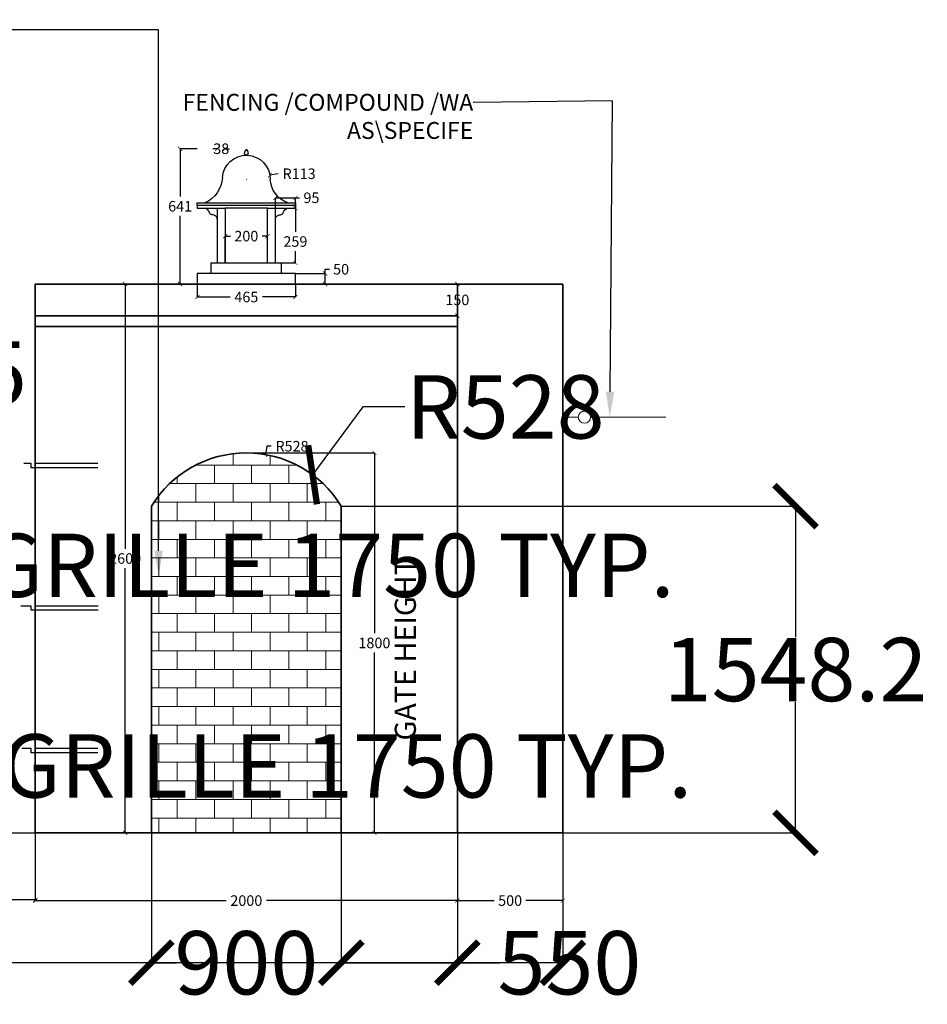
# Model space of a CAD drawing. Units: millimetres. Extents: x 16635 to 28332, y 17519 to 22633.
# Tile 4 of 4: x 24031 to 28332, y 17772 to 22437. Entities that reach past the tile are written whole.
import ezdxf
from ezdxf import colors
from ezdxf.entities.mleader import LeaderData, LeaderLine
from ezdxf.math import Vec2, Vec3

# ---------------------------------------------------------------- set-up
doc = ezdxf.new("R2010")
doc.units = ezdxf.units.MM
doc.header["$MEASUREMENT"] = 0
for name, color, linetype, lineweight in [('A-ANNO-DIMS', 2, 'Continuous', 18), ('A-ANNO-SYMB', 2, 'Continuous', 18), ('A-ANNO-TEXT', 7, 'Continuous', 18), ('A-ELEV-GRAD', 7, 'Continuous', 30), ('A-GATE-HRDW', 3, 'Continuous', 25), ('A-WALL', 7, 'Continuous', 35), ('A-WALL-CHTR', 32, 'Continuous', 25), ('A-WALL-PATT', 8, 'Continuous', 13)]:
    doc.layers.add(name, color=color, linetype=linetype, lineweight=lineweight)
doc.styles.get("Standard").update_dxf_attribs({"font": 'arial.ttf'})
doc.dimstyles.get("Standard").update_dxf_attribs({"dimtxt": 300, "dimasz": 200, "dimexe": 0.18, "dimexo": 0.0625, "dimgap": 0.09, "dimtad": 0, "dimtih": 1, "dimtoh": 1, "dimdec": 0, "dimzin": 0, "dimdsep": 46, "dimtxsty": 'Standard', "dimblk": 'ARCHTICK', "dimcen": 0.09, "dimadec": 0, "dimazin": 0, "dimtfac": 1, "dimtdec": 0, "dimtofl": 0, "dimtmove": 0, "dimatfit": 3, "dimfxl": 1, "dimtolj": 1, "dimtzin": 0, "dimarcsym": 0})

# ---------------------------------------------------------------- blocks, each defined once
blk = doc.blocks.new('_ArchTick')
at = {"color": 0, "linetype": 'ByBlock', "const_width": 0.15}
blk.add_lwpolyline([(-0.5, -0.5), (0.5, 0.5)], dxfattribs=at)
blk = doc.blocks.new('*D1')
at = {"layer": 'A-ANNO-DIMS', "color": 0, "lineweight": -2, "transparency": 16777216}
for p, q in [((25202, 20416), (25195.2, 20376.5)), ((25222, 20416), (25202, 20416)), ((25104.7, 19856.3), (25104.9, 19856.3)), ((25104.8, 19856.3), (25104.8, 19856.4))]:
    blk.add_line(p, q, dxfattribs=at)
at = {"layer": 'Defpoints', "color": 0, "transparency": 16777216}
for p in [(25195.2, 20376.5), (25104.8, 19856.3)]:
    blk.add_point(p, dxfattribs=at)
at = {"layer": 'A-ANNO-DIMS', "color": 0, "lineweight": -2, "transparency": 16777216, "xscale": 20, "yscale": 20, "zscale": 20, "rotation": 260.1400745692449}
blk.add_blockref('_ArchTick', (25195.2, 20376.5), dxfattribs=at)
at = {"layer": 'A-ANNO-DIMS', "color": 0, "transparency": 16777216, "insert": (25321.2, 20416), "char_height": 50, "attachment_point": 5}
blk.add_mtext('\\A1;R528', dxfattribs=at)
blk = doc.blocks.new('*D2')
at = {"layer": 'A-ANNO-DIMS', "color": 0, "lineweight": -2, "transparency": 16777216}
for p, q in [((24872.2, 21825.3), (24790.9, 21825.3)), ((24791.1, 21825.3), (24791.1, 21598.3)), ((24791.1, 21184.3), (24791.1, 21507.3)), ((24872.2, 21184.3), (24790.9, 21184.3))]:
    blk.add_line(p, q, dxfattribs=at)
at = {"layer": 'Defpoints', "color": 0, "transparency": 16777216}
for p in [(24791.1, 21825.3), (24872.3, 21825.3), (24872.3, 21184.3)]:
    blk.add_point(p, dxfattribs=at)
at = {"layer": 'A-ANNO-DIMS', "color": 0, "lineweight": -2, "transparency": 16777216, "xscale": 20, "yscale": 20, "zscale": 20}
for p, rotation in [((24791.1, 21825.3), 90), ((24791.1, 21184.3), 270)]:
    blk.add_blockref('_ArchTick', p, dxfattribs=dict(at, rotation=rotation))
at = {"layer": 'A-ANNO-DIMS', "color": 0, "transparency": 16777216, "insert": (24791.1, 21552.8), "char_height": 50, "attachment_point": 5}
blk.add_mtext('\\A1;641', dxfattribs=at)
blk = doc.blocks.new('*D3')
at = {"layer": 'A-ANNO-DIMS', "color": 0, "lineweight": -2, "transparency": 16777216}
for p, q in [((25255.6, 21706.8), (25216.2, 21700.2)), ((25104.7, 21681.3), (25104.9, 21681.3)), ((25104.8, 21681.3), (25104.8, 21681.4))]:
    blk.add_line(p, q, dxfattribs=at)
at = {"layer": 'Defpoints', "color": 0, "transparency": 16777216}
for p in [(25216.2, 21700.2), (25104.8, 21681.3)]:
    blk.add_point(p, dxfattribs=at)
at = {"layer": 'A-ANNO-DIMS', "color": 0, "lineweight": -2, "transparency": 16777216, "xscale": 20, "yscale": 20, "zscale": 20, "rotation": 189.582500647435}
blk.add_blockref('_ArchTick', (25216.2, 21700.2), dxfattribs=at)
at = {"layer": 'A-ANNO-DIMS', "color": 0, "transparency": 16777216, "insert": (25354.8, 21706.8), "char_height": 50, "attachment_point": 5}
blk.add_mtext('\\A1;R113', dxfattribs=at)
blk = doc.blocks.new('*D4')
at = {"layer": 'A-ANNO-DIMS', "color": 0, "lineweight": -2, "transparency": 16777216}
for p, q in [((24966.8, 21825.3), (24946.8, 21825.3)), ((24966.8, 21825.4), (24966.8, 21825.5)), ((25004.8, 21825.4), (25004.8, 21825.5)), ((25004.8, 21825.3), (25024.8, 21825.3))]:
    blk.add_line(p, q, dxfattribs=at)
at = {"layer": 'Defpoints', "color": 0, "transparency": 16777216}
for p in [(24966.8, 21825.3), (25004.8, 21825.3), (25004.8, 21825.3)]:
    blk.add_point(p, dxfattribs=at)
at = {"layer": 'A-ANNO-DIMS', "color": 0, "lineweight": -2, "transparency": 16777216, "xscale": 20, "yscale": 20, "zscale": 20}
blk.add_blockref('_ArchTick', (24966.8, 21825.3), dxfattribs=at)
at = {"layer": 'A-ANNO-DIMS', "color": 0, "lineweight": -2, "transparency": 16777216, "xscale": 20, "yscale": 20, "zscale": 20, "rotation": 180}
blk.add_blockref('_ArchTick', (25004.8, 21825.3), dxfattribs=at)
at = {"layer": 'A-ANNO-DIMS', "color": 0, "transparency": 16777216, "insert": (24985.8, 21825.3), "char_height": 50, "attachment_point": 5}
blk.add_mtext('\\A1;38', dxfattribs=at)
blk = doc.blocks.new('*D5')
at = {"layer": 'A-ANNO-DIMS', "color": 0, "lineweight": -2, "transparency": 16777216}
for p, q in [((25004.8, 21284.4), (25004.8, 21411.5)), ((25004.8, 21411.3), (25029.2, 21411.3)), ((25204.8, 21411.3), (25180.3, 21411.3)), ((25204.8, 21284.4), (25204.8, 21411.5))]:
    blk.add_line(p, q, dxfattribs=at)
at = {"layer": 'Defpoints', "color": 0, "transparency": 16777216}
for p in [(25204.8, 21411.3), (25004.8, 21284.3), (25204.8, 21284.3)]:
    blk.add_point(p, dxfattribs=at)
at = {"layer": 'A-ANNO-DIMS', "color": 0, "lineweight": -2, "transparency": 16777216, "xscale": 20, "yscale": 20, "zscale": 20, "rotation": 180}
blk.add_blockref('_ArchTick', (25004.8, 21411.3), dxfattribs=at)
at = {"layer": 'A-ANNO-DIMS', "color": 0, "lineweight": -2, "transparency": 16777216, "xscale": 20, "yscale": 20, "zscale": 20}
blk.add_blockref('_ArchTick', (25204.8, 21411.3), dxfattribs=at)
at = {"layer": 'A-ANNO-DIMS', "color": 0, "transparency": 16777216, "insert": (25104.8, 21411.3), "char_height": 50, "attachment_point": 5}
blk.add_mtext('\\A1;200', dxfattribs=at)
blk = doc.blocks.new('*D6')
at = {"layer": 'A-ANNO-DIMS', "color": 0, "lineweight": -2, "transparency": 16777216}
for p, q in [((25337.3, 21234.3), (25478.4, 21234.3)), ((25478.2, 21234.3), (25478.2, 21254.3)), ((25478.2, 21254.3), (25498.2, 21254.3)), ((25478.2, 21184.3), (25478.2, 21234.3)), ((25337.3, 21184.3), (25478.4, 21184.3))]:
    blk.add_line(p, q, dxfattribs=at)
at = {"layer": 'Defpoints', "color": 0, "transparency": 16777216}
for p in [(25337.3, 21234.3), (25478.2, 21234.3), (25337.3, 21184.3)]:
    blk.add_point(p, dxfattribs=at)
at = {"layer": 'A-ANNO-DIMS', "color": 0, "lineweight": -2, "transparency": 16777216, "xscale": 20, "yscale": 20, "zscale": 20}
for p, rotation in [((25478.2, 21234.3), 90), ((25478.2, 21184.3), 270)]:
    blk.add_blockref('_ArchTick', p, dxfattribs=dict(at, rotation=rotation))
at = {"layer": 'A-ANNO-DIMS', "color": 0, "transparency": 16777216, "insert": (25553.9, 21254.3), "char_height": 50, "attachment_point": 5}
blk.add_mtext('\\A1;50', dxfattribs=at)
blk = doc.blocks.new('*D7')
at = {"layer": 'A-ANNO-DIMS', "color": 0, "lineweight": -2, "transparency": 16777216}
for p, q in [((24104.8, 21184.3), (24530.8, 21184.3)), ((24530.6, 21184.3), (24530.6, 19929.9)), ((24530.6, 18584.3), (24530.6, 19838.8)), ((24104.8, 18584.3), (24530.8, 18584.3))]:
    blk.add_line(p, q, dxfattribs=at)
at = {"layer": 'Defpoints', "color": 0, "transparency": 16777216}
for p in [(24104.8, 21184.3), (24104.8, 18584.3), (24530.6, 18584.3)]:
    blk.add_point(p, dxfattribs=at)
at = {"layer": 'A-ANNO-DIMS', "color": 0, "lineweight": -2, "transparency": 16777216, "xscale": 20, "yscale": 20, "zscale": 20}
for p, rotation in [((24530.6, 21184.3), 90), ((24530.6, 18584.3), 270)]:
    blk.add_blockref('_ArchTick', p, dxfattribs=dict(at, rotation=rotation))
at = {"layer": 'A-ANNO-DIMS', "color": 0, "transparency": 16777216, "insert": (24530.6, 19884.3), "char_height": 50, "attachment_point": 5}
blk.add_mtext('\\A1;2600', dxfattribs=at)
blk = doc.blocks.new('*D19')
at = {"layer": 'A-ANNO-DIMS', "color": 0, "lineweight": -2, "transparency": 16777216}
for p, q in [((20204.8, 18584.3), (20204.8, 18267)), ((24104.8, 18584.3), (24104.8, 18267)), ((20204.8, 18267.2), (22060.2, 18267.2)), ((24104.8, 18267.2), (22249.3, 18267.2))]:
    blk.add_line(p, q, dxfattribs=at)
at = {"layer": 'Defpoints', "color": 0, "transparency": 16777216}
for p in [(20204.8, 18584.3), (24104.8, 18584.3), (24104.8, 18267.2)]:
    blk.add_point(p, dxfattribs=at)
at = {"layer": 'A-ANNO-DIMS', "color": 0, "lineweight": -2, "transparency": 16777216, "xscale": 20, "yscale": 20, "zscale": 20, "rotation": 180}
blk.add_blockref('_ArchTick', (20204.8, 18267.2), dxfattribs=at)
at = {"layer": 'A-ANNO-DIMS', "color": 0, "lineweight": -2, "transparency": 16777216, "xscale": 20, "yscale": 20, "zscale": 20}
blk.add_blockref('_ArchTick', (24104.8, 18267.2), dxfattribs=at)
at = {"layer": 'A-ANNO-DIMS', "color": 0, "transparency": 16777216, "insert": (22154.8, 18267.2), "char_height": 50, "attachment_point": 5}
blk.add_mtext('\\A1;3900', dxfattribs=at)
blk = doc.blocks.new('*D20')
at = {"layer": 'A-ANNO-DIMS', "color": 0, "lineweight": -2, "transparency": 16777216}
for p, q in [((24104.8, 18584.3), (24104.8, 18263.6)), ((26104.8, 18584.3), (26104.8, 18263.6)), ((24104.8, 18263.8), (25009.8, 18263.8)), ((26104.8, 18263.8), (25199.8, 18263.8))]:
    blk.add_line(p, q, dxfattribs=at)
at = {"layer": 'Defpoints', "color": 0, "transparency": 16777216}
for p in [(24104.8, 18584.3), (26104.8, 18584.3), (26104.8, 18263.8)]:
    blk.add_point(p, dxfattribs=at)
at = {"layer": 'A-ANNO-DIMS', "color": 0, "lineweight": -2, "transparency": 16777216, "xscale": 20, "yscale": 20, "zscale": 20, "rotation": 180}
blk.add_blockref('_ArchTick', (24104.8, 18263.8), dxfattribs=at)
at = {"layer": 'A-ANNO-DIMS', "color": 0, "lineweight": -2, "transparency": 16777216, "xscale": 20, "yscale": 20, "zscale": 20}
blk.add_blockref('_ArchTick', (26104.8, 18263.8), dxfattribs=at)
at = {"layer": 'A-ANNO-DIMS', "color": 0, "transparency": 16777216, "insert": (25104.8, 18263.8), "char_height": 50, "attachment_point": 5}
blk.add_mtext('\\A1;2000', dxfattribs=at)
blk = doc.blocks.new('*D21')
at = {"layer": 'A-ANNO-DIMS', "color": 0, "lineweight": -2, "transparency": 16777216}
for p, q in [((26104.8, 18584.3), (26104.8, 18263.6)), ((26604.8, 18584.3), (26604.8, 18263.6)), ((26104.8, 18263.8), (26279.6, 18263.8)), ((26604.8, 18263.8), (26429.9, 18263.8))]:
    blk.add_line(p, q, dxfattribs=at)
at = {"layer": 'Defpoints', "color": 0, "transparency": 16777216}
for p in [(26104.8, 18584.3), (26604.8, 18584.3), (26604.8, 18263.8)]:
    blk.add_point(p, dxfattribs=at)
at = {"layer": 'A-ANNO-DIMS', "color": 0, "lineweight": -2, "transparency": 16777216, "xscale": 20, "yscale": 20, "zscale": 20, "rotation": 180}
blk.add_blockref('_ArchTick', (26104.8, 18263.8), dxfattribs=at)
at = {"layer": 'A-ANNO-DIMS', "color": 0, "lineweight": -2, "transparency": 16777216, "xscale": 20, "yscale": 20, "zscale": 20}
blk.add_blockref('_ArchTick', (26604.8, 18263.8), dxfattribs=at)
at = {"layer": 'A-ANNO-DIMS', "color": 0, "transparency": 16777216, "insert": (26354.8, 18263.8), "char_height": 50, "attachment_point": 5}
blk.add_mtext('\\A1;500', dxfattribs=at)
blk = doc.blocks.new('*D22')
at = {"layer": 'A-ANNO-DIMS', "color": 0, "lineweight": -2, "transparency": 16777216}
for p, q in [((25104.8, 20384.3), (25711.9, 20384.3)), ((25711.8, 20384.3), (25711.8, 19529.9)), ((25711.8, 18584.3), (25711.8, 19438.8)), ((25104.8, 18584.3), (25711.9, 18584.3))]:
    blk.add_line(p, q, dxfattribs=at)
at = {"layer": 'Defpoints', "color": 0, "transparency": 16777216}
for p in [(25104.8, 20384.3), (25104.8, 18584.3), (25711.8, 18584.3)]:
    blk.add_point(p, dxfattribs=at)
at = {"layer": 'A-ANNO-DIMS', "color": 0, "lineweight": -2, "transparency": 16777216, "xscale": 20, "yscale": 20, "zscale": 20}
for p, rotation in [((25711.8, 20384.3), 90), ((25711.8, 18584.3), 270)]:
    blk.add_blockref('_ArchTick', p, dxfattribs=dict(at, rotation=rotation))
at = {"layer": 'A-ANNO-DIMS', "color": 0, "transparency": 16777216, "insert": (25711.8, 19484.3), "char_height": 50, "attachment_point": 5}
blk.add_mtext('\\A1;1800', dxfattribs=at)
blk = doc.blocks.new('*D25')
at = {"layer": 'A-ANNO-DIMS', "color": 0, "lineweight": -2, "transparency": 16777216}
for p, q in [((26104.7, 21184.3), (26104.6, 21184.3)), ((26104.8, 21184.3), (26104.8, 21154.9)), ((26104.8, 21034.3), (26104.8, 21063.8)), ((26104.7, 21034.3), (26104.6, 21034.3))]:
    blk.add_line(p, q, dxfattribs=at)
at = {"layer": 'Defpoints', "color": 0, "transparency": 16777216}
for p in [(26104.8, 21184.3), (26104.8, 21034.3), (26104.8, 21034.3)]:
    blk.add_point(p, dxfattribs=at)
at = {"layer": 'A-ANNO-DIMS', "color": 0, "lineweight": -2, "transparency": 16777216, "xscale": 20, "yscale": 20, "zscale": 20}
for p, rotation in [((26104.8, 21184.3), 90), ((26104.8, 21034.3), 270)]:
    blk.add_blockref('_ArchTick', p, dxfattribs=dict(at, rotation=rotation))
at = {"layer": 'A-ANNO-DIMS', "color": 0, "transparency": 16777216, "insert": (26104.8, 21109.3), "char_height": 50, "attachment_point": 5}
blk.add_mtext('\\A1;150', dxfattribs=at)
blk = doc.blocks.new('*D26')
at = {"layer": 'A-ANNO-DIMS', "color": 0, "lineweight": -2, "transparency": 16777216}
for p, q in [((24872.3, 21184.3), (24872.3, 21122.9)), ((25337.3, 21184.3), (25337.3, 21122.9)), ((24872.3, 21123), (25028.3, 21123)), ((25337.3, 21123), (25181.2, 21123))]:
    blk.add_line(p, q, dxfattribs=at)
at = {"layer": 'Defpoints', "color": 0, "transparency": 16777216}
for p in [(24872.3, 21184.3), (25337.3, 21184.3), (25337.3, 21123)]:
    blk.add_point(p, dxfattribs=at)
at = {"layer": 'A-ANNO-DIMS', "color": 0, "lineweight": -2, "transparency": 16777216, "xscale": 20, "yscale": 20, "zscale": 20, "rotation": 180}
blk.add_blockref('_ArchTick', (24872.3, 21123), dxfattribs=at)
at = {"layer": 'A-ANNO-DIMS', "color": 0, "lineweight": -2, "transparency": 16777216, "xscale": 20, "yscale": 20, "zscale": 20}
blk.add_blockref('_ArchTick', (25337.3, 21123), dxfattribs=at)
at = {"layer": 'A-ANNO-DIMS', "color": 0, "transparency": 16777216, "insert": (25104.8, 21123), "char_height": 50, "attachment_point": 5}
blk.add_mtext('\\A1;465', dxfattribs=at)
blk = doc.blocks.new('*D27')
at = {"layer": 'A-ANNO-DIMS', "color": 0, "lineweight": -2, "transparency": 16777216}
for p, q in [((25242.8, 21543.4), (25242.8, 21593.1)), ((25242.8, 21593), (25337.3, 21593)), ((25337.3, 21543.4), (25337.3, 21593.1)), ((25337.3, 21593), (25357.3, 21593))]:
    blk.add_line(p, q, dxfattribs=at)
at = {"layer": 'Defpoints', "color": 0, "transparency": 16777216}
for p in [(25337.3, 21593), (25242.8, 21543.3), (25337.3, 21543.3)]:
    blk.add_point(p, dxfattribs=at)
at = {"layer": 'A-ANNO-DIMS', "color": 0, "lineweight": -2, "transparency": 16777216, "xscale": 20, "yscale": 20, "zscale": 20, "rotation": 180}
blk.add_blockref('_ArchTick', (25242.8, 21593), dxfattribs=at)
at = {"layer": 'A-ANNO-DIMS', "color": 0, "lineweight": -2, "transparency": 16777216, "xscale": 20, "yscale": 20, "zscale": 20}
blk.add_blockref('_ArchTick', (25337.3, 21593), dxfattribs=at)
at = {"layer": 'A-ANNO-DIMS', "color": 0, "transparency": 16777216, "insert": (25413.3, 21593), "char_height": 50, "attachment_point": 5}
blk.add_mtext('\\A1;95', dxfattribs=at)
blk = doc.blocks.new('*D29')
at = {"layer": 'A-ANNO-DIMS', "color": 0, "lineweight": -2, "transparency": 16777216}
for p, q in [((25204.8, 21543.3), (25337.5, 21543.3)), ((25337.3, 21543.3), (25337.3, 21431.2)), ((25337.3, 21284.3), (25337.3, 21340.2)), ((25204.8, 21284.3), (25337.5, 21284.3))]:
    blk.add_line(p, q, dxfattribs=at)
at = {"layer": 'Defpoints', "color": 0, "transparency": 16777216}
for p in [(25204.8, 21543.3), (25204.8, 21284.3), (25337.3, 21284.3)]:
    blk.add_point(p, dxfattribs=at)
at = {"layer": 'A-ANNO-DIMS', "color": 0, "lineweight": -2, "transparency": 16777216, "xscale": 20, "yscale": 20, "zscale": 20}
for p, rotation in [((25337.3, 21543.3), 90), ((25337.3, 21284.3), 270)]:
    blk.add_blockref('_ArchTick', p, dxfattribs=dict(at, rotation=rotation))
at = {"layer": 'A-ANNO-DIMS', "color": 0, "transparency": 16777216, "insert": (25337.3, 21385.7), "char_height": 50, "attachment_point": 5}
blk.add_mtext('\\A1;259', dxfattribs=at)
blk = doc.blocks.new('STONE-CHHATRI-ELEV')
for p, q in [((465, 384), (0, 384)), ((0, 384), (0, 359)), ((465, 371.5), (465, 384)), ((0, 371.5), (465, 371.5)), ((132.5, 359), (0, 359)), ((94.5, 100), (94.5, 359)), ((132.5, 100), (132.5, 359)), ((132.5, 359), (332.5, 359)), ((332.5, 359), (332.5, 100)), ((465, 359), (332.5, 359)), ((370.5, 359), (370.5, 100)), ((465, 371.5), (465, 359)), ((398.8, 100), (66.3, 100)), ((66.3, 50), (66.3, 100)), ((398.8, 50), (398.8, 100)), ((0, 0), (0, 50)), ((0, 50), (465, 50)), ((465, 50), (465, 0))]:
    blk.add_line(p, q)
for points in [[(223.5, 618.7, -0.258687), (233, 636.9, -0.244698), (241.5, 619.3, -0.244698)], [(94.5, 307.9, 0.449164), (70.8, 327.5, -0.238561), (57.7, 338.5, 0.309009), (37.1, 359, -1.219644)], [(370.5, 307.9, -0.449164), (394.2, 327.5, 0.238561), (407.3, 338.5, -0.309009), (427.9, 359, 1.219644)]]:
    blk.add_lwpolyline(points, format="xyb")
for centre, radius, start, end in [((232.5, 497), 113, 3.6245, 179.9064), ((232.5, 619), 9.02, 180.1799, 1.9928), ((-8.8, 504.3), 128.5, 290.6287, 356.8247), ((488.3, 514.4), 143.4, 184.0947, 245.367)]:
    blk.add_arc(centre, radius, start, end)
blk = doc.blocks.new('GATE-JAMB-ANCHOR-SET')
for p, q in [((0.2, 1370), (297.2, 1370)), ((317.2, 1350), (317.2, 1370)), ((317.2, 1370), (351.9, 1370)), ((0.2, 1350), (297.2, 1350)), ((297.2, 1350), (317.2, 1350)), ((0, 694.8), (297, 694.8)), ((0, 674.8), (297, 674.8)), ((297, 674.8), (317, 674.8)), ((317, 674.8), (317, 694.8)), ((317, 694.8), (365.3, 694.8)), ((0.2, 20), (297.2, 20)), ((317.2, 0), (317.2, 20)), ((317.2, 20), (360.9, 20)), ((0.2, 0), (297.2, 0)), ((297.2, 0), (317.2, 0))]:
    blk.add_line(p, q)
blk = doc.blocks.new('*D43')
at = {"layer": 'A-ANNO-DIMS', "color": 0, "lineweight": -2, "transparency": 16777216}
for p, q in [((20304.8, 19164.3), (20304.8, 18901.7)), ((22054.8, 19164.3), (22054.8, 18901.7)), ((20304.8, 18901.8), (22054.8, 18901.8)), ((22054.8, 18901.8), (22254.8, 18901.8))]:
    blk.add_line(p, q, dxfattribs=at)
at = {"layer": 'Defpoints', "color": 0, "transparency": 16777216}
for p in [(20304.8, 19164.3), (22054.8, 19164.3), (22054.8, 18901.8)]:
    blk.add_point(p, dxfattribs=at)
at = {"layer": 'A-ANNO-DIMS', "color": 0, "lineweight": -2, "transparency": 16777216, "xscale": 200, "yscale": 200, "zscale": 200, "rotation": 180}
blk.add_blockref('_ArchTick', (20304.8, 18901.8), dxfattribs=at)
at = {"layer": 'A-ANNO-DIMS', "color": 0, "lineweight": -2, "transparency": 16777216, "xscale": 200, "yscale": 200, "zscale": 200}
blk.add_blockref('_ArchTick', (22054.8, 18901.8), dxfattribs=at)
at = {"layer": 'A-ANNO-DIMS', "color": 0, "transparency": 16777216, "insert": (24841.7, 18901.8), "char_height": 300, "attachment_point": 5}
blk.add_mtext('\\A1;LOWER GRILLE 1750 TYP.', dxfattribs=at)
blk = doc.blocks.new('*D45')
at = {"layer": 'A-ANNO-DIMS', "color": 0, "lineweight": -2, "transparency": 16777216}
for p, q in [((20304.8, 20114.3), (20304.8, 19851.7)), ((22054.8, 20114.3), (22054.8, 19851.7)), ((20304.8, 19851.8), (22054.8, 19851.8)), ((22054.8, 19851.8), (22254.8, 19851.8))]:
    blk.add_line(p, q, dxfattribs=at)
at = {"layer": 'Defpoints', "color": 0, "transparency": 16777216}
for p in [(20304.8, 20114.3), (22054.8, 20114.3), (22054.8, 19851.8)]:
    blk.add_point(p, dxfattribs=at)
at = {"layer": 'A-ANNO-DIMS', "color": 0, "lineweight": -2, "transparency": 16777216, "xscale": 200, "yscale": 200, "zscale": 200, "rotation": 180}
blk.add_blockref('_ArchTick', (20304.8, 19851.8), dxfattribs=at)
at = {"layer": 'A-ANNO-DIMS', "color": 0, "lineweight": -2, "transparency": 16777216, "xscale": 200, "yscale": 200, "zscale": 200}
blk.add_blockref('_ArchTick', (22054.8, 19851.8), dxfattribs=at)
at = {"layer": 'A-ANNO-DIMS', "color": 0, "transparency": 16777216, "insert": (24794.1, 19851.8), "char_height": 300, "attachment_point": 5}
blk.add_mtext('\\A1;UPPER GRILLE 1750 TYP.', dxfattribs=at)
blk = doc.blocks.new('*D51')
at = {"layer": 'A-ANNO-DIMS', "color": 0, "lineweight": -2, "transparency": 16777216}
for p, q in [((17704.8, 18584.3), (17704.8, 17969.2)), ((26604.8, 18584.3), (26604.8, 17969.2)), ((17704.8, 17969.3), (21707, 17969.3)), ((26604.8, 17969.3), (22602.5, 17969.3))]:
    blk.add_line(p, q, dxfattribs=at)
at = {"layer": 'Defpoints', "color": 0, "transparency": 16777216}
for p in [(17704.8, 18584.3), (26604.8, 18584.3), (26604.8, 17969.3)]:
    blk.add_point(p, dxfattribs=at)
at = {"layer": 'A-ANNO-DIMS', "color": 0, "lineweight": -2, "transparency": 16777216, "xscale": 200, "yscale": 200, "zscale": 200, "rotation": 180}
blk.add_blockref('_ArchTick', (17704.8, 17969.3), dxfattribs=at)
at = {"layer": 'A-ANNO-DIMS', "color": 0, "lineweight": -2, "transparency": 16777216, "xscale": 200, "yscale": 200, "zscale": 200}
blk.add_blockref('_ArchTick', (26604.8, 17969.3), dxfattribs=at)
at = {"layer": 'A-ANNO-DIMS', "color": 0, "transparency": 16777216, "insert": (22154.8, 17969.3), "char_height": 300, "attachment_point": 5}
blk.add_mtext('\\A1;8900', dxfattribs=at)
blk = doc.blocks.new('*D54')
at = {"layer": 'A-ANNO-DIMS', "color": 0, "lineweight": -2, "transparency": 16777216}
for p, q in [((25554.8, 20132.5), (27707.3, 20132.5)), ((27707.2, 20132.5), (27707.2, 19511.7)), ((27707.2, 18584.3), (27707.2, 19205.2)), ((25554.8, 18584.3), (27707.3, 18584.3))]:
    blk.add_line(p, q, dxfattribs=at)
at = {"layer": 'Defpoints', "color": 0, "transparency": 16777216}
for p in [(25554.8, 20132.5), (27707.2, 20132.5), (25554.8, 18584.3)]:
    blk.add_point(p, dxfattribs=at)
at = {"layer": 'A-ANNO-DIMS', "color": 0, "lineweight": -2, "transparency": 16777216, "xscale": 200, "yscale": 200, "zscale": 200}
for p, rotation in [((27707.2, 20132.5), 90), ((27707.2, 18584.3), 270)]:
    blk.add_blockref('_ArchTick', p, dxfattribs=dict(at, rotation=rotation))
at = {"layer": 'A-ANNO-DIMS', "color": 0, "transparency": 16777216, "insert": (27707.2, 19358.4), "char_height": 300, "attachment_point": 5}
blk.add_mtext('\\A1;1548.2', dxfattribs=at)
blk = doc.blocks.new('*D57')
at = {"layer": 'A-ANNO-DIMS', "color": 0, "lineweight": -2, "transparency": 16777216}
for p, q in [((25554.8, 18584.3), (25554.8, 17969.2)), ((26104.8, 18584.3), (26104.8, 17969.2)), ((25554.8, 17969.3), (26104.8, 17969.3)), ((26104.8, 17969.3), (26304.8, 17969.3))]:
    blk.add_line(p, q, dxfattribs=at)
at = {"layer": 'Defpoints', "color": 0, "transparency": 16777216}
for p in [(25554.8, 18584.3), (26104.8, 18584.3), (26104.8, 17969.3)]:
    blk.add_point(p, dxfattribs=at)
at = {"layer": 'A-ANNO-DIMS', "color": 0, "lineweight": -2, "transparency": 16777216, "xscale": 200, "yscale": 200, "zscale": 200, "rotation": 180}
blk.add_blockref('_ArchTick', (25554.8, 17969.3), dxfattribs=at)
at = {"layer": 'A-ANNO-DIMS', "color": 0, "lineweight": -2, "transparency": 16777216, "xscale": 200, "yscale": 200, "zscale": 200}
blk.add_blockref('_ArchTick', (26104.8, 17969.3), dxfattribs=at)
at = {"layer": 'A-ANNO-DIMS', "color": 0, "transparency": 16777216, "insert": (26635.8, 17969.3), "char_height": 300, "attachment_point": 5}
blk.add_mtext('\\A1;550', dxfattribs=at)
blk = doc.blocks.new('*D58')
at = {"layer": 'A-ANNO-DIMS', "color": 0, "lineweight": -2, "transparency": 16777216}
for p, q in [((24654.8, 18584.3), (24654.8, 17969.2)), ((25554.8, 18584.3), (25554.8, 17969.2)), ((24654.8, 17969.3), (24773.8, 17969.3)), ((25554.8, 17969.3), (25435.8, 17969.3))]:
    blk.add_line(p, q, dxfattribs=at)
at = {"layer": 'Defpoints', "color": 0, "transparency": 16777216}
for p in [(24654.8, 18584.3), (25554.8, 18584.3), (25554.8, 17969.3)]:
    blk.add_point(p, dxfattribs=at)
at = {"layer": 'A-ANNO-DIMS', "color": 0, "lineweight": -2, "transparency": 16777216, "xscale": 200, "yscale": 200, "zscale": 200, "rotation": 180}
blk.add_blockref('_ArchTick', (24654.8, 17969.3), dxfattribs=at)
at = {"layer": 'A-ANNO-DIMS', "color": 0, "lineweight": -2, "transparency": 16777216, "xscale": 200, "yscale": 200, "zscale": 200}
blk.add_blockref('_ArchTick', (25554.8, 17969.3), dxfattribs=at)
at = {"layer": 'A-ANNO-DIMS', "color": 0, "transparency": 16777216, "insert": (25104.8, 17969.3), "char_height": 300, "attachment_point": 5}
blk.add_mtext('\\A1;900', dxfattribs=at)
blk = doc.blocks.new('*D63')
at = {"layer": 'A-ANNO-DIMS', "color": 0, "lineweight": -2, "transparency": 16777216}
for p, q in [((25656.5, 20602.5), (25418.7, 20280.9)), ((25856.5, 20602.5), (25656.5, 20602.5)), ((25104.7, 19856.3), (25104.9, 19856.3)), ((25104.8, 19856.3), (25104.8, 19856.4))]:
    blk.add_line(p, q, dxfattribs=at)
at = {"layer": 'Defpoints', "color": 0, "transparency": 16777216}
for p in [(25418.7, 20280.9), (25104.8, 19856.3)]:
    blk.add_point(p, dxfattribs=at)
at = {"layer": 'A-ANNO-DIMS', "color": 0, "lineweight": -2, "transparency": 16777216, "xscale": 200, "yscale": 200, "zscale": 200, "rotation": 233.52236858087}
blk.add_blockref('_ArchTick', (25418.7, 20280.9), dxfattribs=at)
at = {"layer": 'A-ANNO-DIMS', "color": 0, "transparency": 16777216, "insert": (26331.8, 20602.5), "char_height": 300, "attachment_point": 5}
blk.add_mtext('\\A1;R528', dxfattribs=at)
blk = doc.blocks.new('*D70')
at = {"layer": 'A-ANNO-DIMS', "color": 0, "lineweight": -2, "transparency": 16777216}
for p, q in [((21971.5, 20762.6), (21591.1, 20639)), ((22171.5, 20762.6), (21971.5, 20762.6)), ((21179.7, 20505.3), (21179.9, 20505.3)), ((21179.8, 20505.3), (21179.8, 20505.4))]:
    blk.add_line(p, q, dxfattribs=at)
at = {"layer": 'Defpoints', "color": 0, "transparency": 16777216}
for p in [(21591.1, 20639), (21179.8, 20505.3)]:
    blk.add_point(p, dxfattribs=at)
at = {"layer": 'A-ANNO-DIMS', "color": 0, "lineweight": -2, "transparency": 16777216, "xscale": 200, "yscale": 200, "zscale": 200, "rotation": 198.0002935108227}
blk.add_blockref('_ArchTick', (21591.1, 20639), dxfattribs=at)
at = {"layer": 'A-ANNO-DIMS', "color": 0, "transparency": 16777216, "insert": (23147.3, 20762.6), "char_height": 300, "attachment_point": 5}
blk.add_mtext('\\A1;2X R432.5', dxfattribs=at)

msp = doc.modelspace()

# ---------------------------------------------------------------- hatches: boundary and pattern name
at = {"layer": 'A-WALL-PATT'}
h = msp.add_hatch(dxfattribs=at)
h.set_pattern_fill('AR-B816', color=256, scale=11)
h.set_pattern_definition([(0, (15185.615, 17862.945), (0, 88), []), (90, (15185.615, 17862.945), (-88, 88), [88, -88])])
h.paths.add_polyline_path([(24654.77, 20132.544), (24654.77, 18584.349), (25554.77, 18584.349), (25554.77, 20132.544, 0.55956537)])

# ---------------------------------------------------------------- linework, layer by layer
at = {"layer": 'A-ANNO-SYMB'}
for p, q in [((26604.77, 20553.851), (26677.968, 20553.851)), ((26735.87, 20553.851), (27092.159, 20553.851))]:
    msp.add_line(p, q, dxfattribs=at)
msp.add_circle((26706.919, 20553.851), 28.951, dxfattribs=at)
at = {"layer": 'A-ELEV-GRAD'}
msp.add_line((20204.77, 18584.349), (24104.77, 18584.349), dxfattribs=at)
at = {"layer": 'A-WALL'}
for p, q in [((24104.77, 18584.349), (24104.77, 21184.349)), ((24104.77, 21184.349), (26604.77, 21184.349)), ((26104.77, 18584.349), (26104.77, 21184.349)), ((26604.77, 18584.349), (26604.77, 21184.349)), ((24104.77, 21034.349), (26104.77, 21034.349)), ((24104.77, 20983.349), (26104.77, 20983.349)), ((24654.77, 18584.349), (24654.77, 20132.544)), ((25554.77, 18584.349), (25554.77, 20132.544)), ((24104.77, 18584.349), (26604.77, 18584.349))]:
    msp.add_line(p, q, dxfattribs=at)
msp.add_arc((25104.77, 19856.349), 528, 31.540269, 148.459731, dxfattribs=at)

# ---------------------------------------------------------------- block references
at = {"layer": 'A-GATE-HRDW', "extrusion": (0, 0, -1), "zscale": -1}
msp.add_blockref('GATE-JAMB-ANCHOR-SET', (-24401.971, 18964.349), dxfattribs=at)
at = {"layer": 'A-WALL-CHTR', "extrusion": (0, 0, -1), "zscale": -1}
msp.add_blockref('STONE-CHHATRI-ELEV', (-25337.271, 21184.349), dxfattribs=at)

# ---------------------------------------------------------------- texts
at = {"layer": 'A-ANNO-TEXT'}
msp.add_text('GATE HEIGHT', height=100, rotation=90, dxfattribs=at).set_placement((25908.148, 19022.025))

# ---------------------------------------------------------------- dimensions: what is measured, and where the dimension line sits
at = {"layer": 'A-ANNO-DIMS'}
for base, p1, p2, picture, middle in [((24791.086, 21825.349), (24872.27, 21184.349), (24872.27, 21825.349), '*D2', (24791.086, 21552.794)), ((25337.27, 21284.349), (25204.77, 21543.349), (25204.77, 21284.349), '*D29', (25337.27, 21385.717)), ((26104.77, 21034.349), (26104.77, 21184.349), (26104.77, 21034.349), '*D25', (26104.77, 21109.349))]:
    dim = msp.add_linear_dim(base=base, p1=p1, p2=p2, angle=90, dimstyle='Standard', override={"dimtxt": 50, "dimasz": 20, "dimgap": 20, "dimclrd": 0, "dimclre": 0, "dimclrt": 0}, dxfattribs=at)
    dim.commit()
    dim.dimension.update_dxf_attribs({"geometry": picture, "text_midpoint": middle, "dimtype": 160})
for base, p1, p2, picture, middle in [((25004.77, 21825.349), (24966.77, 21825.349), (25004.77, 21825.349), '*D4', (24985.77, 21825.349)), ((25204.77, 21411.271), (25004.77, 21284.349), (25204.77, 21284.349), '*D5', (25104.77, 21411.271))]:
    dim = msp.add_linear_dim(base=base, p1=p1, p2=p2, dimstyle='Standard', override={"dimtxt": 50, "dimasz": 20, "dimgap": 20, "dimclrd": 0, "dimclre": 0, "dimclrt": 0}, dxfattribs=at)
    dim.commit()
    dim.dimension.update_dxf_attribs({"geometry": picture, "text_midpoint": middle, "dimtype": 160})
for center, mpoint, override, picture, middle in [((25104.77, 21681.349), (25216.194, 21700.159), {"dimtxt": 50, "dimasz": 20, "dimgap": 20, "dimclrd": 0, "dimclre": 0, "dimclrt": 0}, '*D3', (25354.796, 21706.818)), ((25104.77, 19856.349), (25418.671, 20280.908), {"dimdec": 0, "dimlfac": 1, "dimrnd": 0, "dimzin": 0, "dimdsep": 46, "dimlunit": 2}, '*D63', (26331.837, 20602.543)), ((25104.77, 19856.349), (25195.185, 20376.55), {"dimtxt": 50, "dimasz": 20, "dimgap": 20, "dimclrd": 0, "dimclre": 0, "dimclrt": 0}, '*D1', (25321.247, 20415.959))]:
    dim = msp.add_radius_dim(center=center, mpoint=mpoint, dimstyle='Standard', override=override, dxfattribs=at)
    dim.commit()
    dim.dimension.update_dxf_attribs({"geometry": picture, "text_midpoint": middle})
for base, p1, p2, override, picture, middle in [((25337.270299627, 21592.969397776), (25242.770299627, 21543.348549447), (25337.270299627, 21543.348549447), {"dimtxt": 50, "dimasz": 20, "dimgap": 20, "dimclrd": 0, "dimclre": 0, "dimclrt": 0}, '*D27', (25413.269617499, 21592.969397776)), ((25337.27, 21123.04), (24872.27, 21184.349), (25337.27, 21184.349), {"dimtxt": 50, "dimasz": 20, "dimgap": 20, "dimclrd": 0, "dimclre": 0, "dimclrt": 0}, '*D26', (25104.77, 21123.04)), ((26604.77, 17969.349), (17704.77, 18584.349), (26604.77, 18584.349), {"dimdec": 0, "dimlfac": 1, "dimrnd": 0, "dimzin": 0, "dimdsep": 46, "dimlunit": 2}, '*D51', (22154.77, 17969.349)), ((24104.77, 18267.158), (20204.77, 18584.349), (24104.77, 18584.349), {"dimtxt": 50, "dimasz": 20, "dimgap": 20, "dimclrd": 0, "dimclre": 0, "dimclrt": 0}, '*D19', (22154.77, 18267.158)), ((26104.77, 18263.824), (24104.77, 18584.349), (26104.77, 18584.349), {"dimtxt": 50, "dimasz": 20, "dimgap": 20, "dimclrd": 0, "dimclre": 0, "dimclrt": 0}, '*D20', (25104.77, 18263.824)), ((25554.77, 17969.349), (24654.77, 18584.349), (25554.77, 18584.349), {"dimdec": 0, "dimlfac": 1, "dimrnd": 0, "dimzin": 0, "dimdsep": 46, "dimlunit": 2}, '*D58', (25104.77, 17969.349)), ((26104.77, 17969.349), (25554.77, 18584.349), (26104.77, 18584.349), {"dimdec": 0, "dimlfac": 1, "dimrnd": 0, "dimzin": 0, "dimdsep": 46, "dimlunit": 2}, '*D57', (26635.761, 17969.349)), ((26604.77, 18263.824), (26104.77, 18584.349), (26604.77, 18584.349), {"dimtxt": 50, "dimasz": 20, "dimgap": 20, "dimclrd": 0, "dimclre": 0, "dimclrt": 0}, '*D21', (26354.77, 18263.824))]:
    dim = msp.add_linear_dim(base=base, p1=p1, p2=p2, dimstyle='Standard', override=override, dxfattribs=at)
    dim.commit()
    dim.dimension.update_dxf_attribs({"geometry": picture, "text_midpoint": middle})
for base, p1, p2, override, picture, middle in [((25478.214, 21234.349), (25337.27, 21184.349), (25337.27, 21234.349), {"dimtxt": 50, "dimasz": 20, "dimgap": 20, "dimclrd": 0, "dimclre": 0, "dimclrt": 0}, '*D6', (25553.94, 21254.349)), ((24530.604, 18584.349), (24104.77, 21184.349), (24104.77, 18584.349), {"dimtxt": 50, "dimasz": 20, "dimgap": 20, "dimclrd": 0, "dimclre": 0, "dimclrt": 0}, '*D7', (24530.604, 19884.349)), ((25711.767, 18584.349), (25104.77, 20384.349), (25104.77, 18584.349), {"dimtxt": 50, "dimasz": 20, "dimgap": 20, "dimclrd": 0, "dimclre": 0, "dimclrt": 0}, '*D22', (25711.767, 19484.349)), ((27707.159, 20132.544), (25554.77, 18584.349), (25554.77, 20132.544), {"dimdec": 1, "dimlfac": 1, "dimrnd": 0, "dimzin": 0, "dimdsep": 46, "dimlunit": 2}, '*D54', (27707.159, 19358.446))]:
    dim = msp.add_linear_dim(base=base, p1=p1, p2=p2, angle=90, dimstyle='Standard', override=override, dxfattribs=at)
    dim.commit()
    dim.dimension.update_dxf_attribs({"geometry": picture, "text_midpoint": middle})
dim = msp.add_radius_dim(center=(21179.77, 20505.349), mpoint=(21591.102, 20639.001), text='2X <>', dimstyle='Standard', override={"dimdec": 1, "dimlfac": 1, "dimrnd": 0, "dimzin": 0, "dimdsep": 46, "dimlunit": 2}, dxfattribs=at)
dim.commit()
dim.dimension.update_dxf_attribs({"geometry": '*D70', "text_midpoint": (23147.33, 20762.609)})
for base, p1, p2, text, picture, middle in [((22054.77, 19851.849), (20304.77, 20114.349), (22054.77, 20114.349), 'UPPER GRILLE <> TYP.', '*D45', (24794.117, 19851.849)), ((22054.77, 18901.849), (20304.77, 19164.349), (22054.77, 19164.349), 'LOWER GRILLE <> TYP.', '*D43', (24841.695, 18901.849))]:
    dim = msp.add_linear_dim(base=base, p1=p1, p2=p2, text=text, dimstyle='Standard', override={"dimdec": 0, "dimlfac": 1, "dimrnd": 0, "dimzin": 0, "dimdsep": 46, "dimlunit": 2}, dxfattribs=at)
    dim.commit()
    dim.dimension.update_dxf_attribs({"geometry": picture, "text_midpoint": middle})

# ---------------------------------------------------------------- leaders
at = {"layer": 'A-ANNO-TEXT'}
ml = msp.add_multileader_mtext('Standard', dxfattribs=at)
ml.set_content('SAND\\\\STONE\\\\TIL\\PCLADDIND', color=256)
ml.set_leader_properties()
ml.build(insert=Vec2(0, 0))
ml.multileader.update_dxf_attribs({"dogleg_length": 0.36, "arrow_head_size": 120})
ctx = ml.context
ctx.base_point, ctx.char_height, ctx.arrow_head_size, ctx.landing_gap_size, ctx.plane_origin = Vec3(22967.113, 22389.231), 80, 120, 0.09, Vec3(23877.721, 22389.231)
ctx.text_align_type = 2
notes = []
notes.append((ctx, [(0, (1, 1, 0), (23877.721, 22389.231), (-1, 0), 0.36, [(0, [(24689.11, 19800.774), (24689.11, 22389.231)], 0, [])])]))
ctx.mtext.insert, ctx.mtext.alignment, ctx.mtext.flow_direction = Vec3(23877.271, 22429.914), 3, 5
ml = msp.add_multileader_mtext('Standard', dxfattribs=at)
ml.set_content('FENCING /COMPOUND /WA\\PAS\\\\SPECIFE', color=256)
ml.set_leader_properties()
ml.build(insert=Vec2(0, 0))
ml.multileader.update_dxf_attribs({"dogleg_length": 0.36, "arrow_head_size": 120})
ctx = ml.context
ctx.base_point, ctx.char_height, ctx.arrow_head_size, ctx.landing_gap_size, ctx.plane_origin = Vec3(24717.823, 22044.572), 80, 120, 0.09, Vec3(26180.846, 22044.572)
ctx.text_align_type = 2
notes.append((ctx, [(0, (1, 1, 0), (26180.846, 22044.572), (-1, 0), 0.36, [(0, [(26827.299, 20553.851), (26840.321, 22051.702)], 0, [])])]))
ctx.mtext.insert, ctx.mtext.alignment, ctx.mtext.flow_direction = Vec3(26180.396, 22085.254), 3, 5
for ctx, leaders in notes:
    for number, flags, end, landing, length, lines in leaders:
        leader = LeaderData()
        leader.index, (leader.has_last_leader_line, leader.has_dogleg_vector, leader.attachment_direction) = number, flags
        leader.last_leader_point, leader.dogleg_vector, leader.dogleg_length = Vec3(end), Vec3(landing), length
        for number, points, colour, breaks in lines:
            line = LeaderLine()
            line.index, line.vertices, line.color, line.breaks = number, Vec3.list(points), colors.encode_raw_color(colour), breaks
            leader.lines.append(line)
        ctx.leaders.append(leader)

doc.saveas('drawing.dxf')
